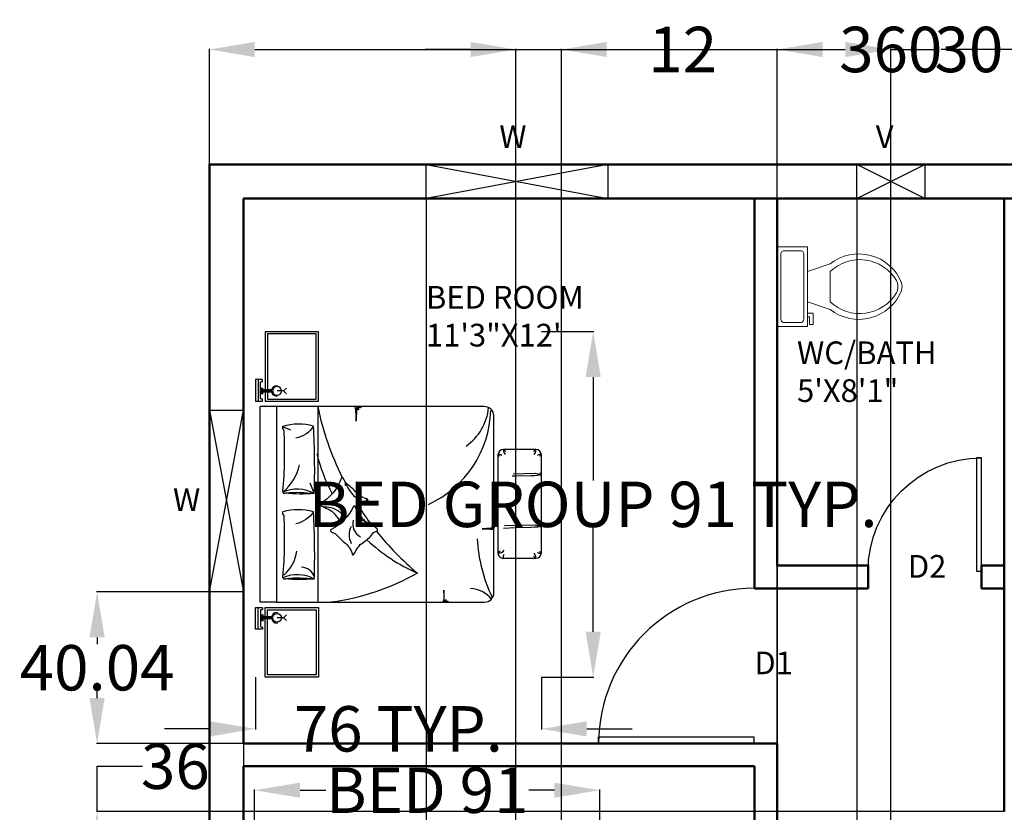
# Model space of a CAD drawing. Units: inches. Extents: x -77 to 516, y -119 to 536.
# Tile 7 of 11: x -36 to 224, y 323 to 533. Entities that reach past the tile are written whole.
import ezdxf

# ---------------------------------------------------------------- set-up
doc = ezdxf.new("R2010")
doc.units = ezdxf.units.IN
doc.header["$MEASUREMENT"] = 0
for name, color, linetype, lineweight in [('A-ANNO-DIMS', 2, 'Continuous', 18), ('A-AREA-IDEN', 170, 'Continuous', 25), ('A-FLOR-FIXT', 9, 'Continuous', 18), ('doors', 6, 'Continuous', 25), ('furniture', 119, 'Continuous', 18), ('text', 170, 'Continuous', 18), ('walls', 40, 'Continuous', 50), ('windows', 1, 'Continuous', 25)]:
    doc.layers.add(name, color=color, linetype=linetype, lineweight=lineweight)
for name, color, linetype in [('CEIL', 4, 'Continuous'), ('ELEC', 4, 'Continuous'), ('FUR', 42, 'Continuous'), ('wood', 26, 'Continuous')]:
    doc.layers.add(name, color=color, linetype=linetype)
doc.styles.get("Standard").update_dxf_attribs({"font": 'arial.ttf'})
doc.dimstyles.get("Standard").update_dxf_attribs({"dimtxt": 12, "dimasz": 12, "dimexe": 0.18, "dimexo": 0.0625, "dimgap": 0.09, "dimtad": 0, "dimtih": 1, "dimtoh": 1, "dimdec": 1, "dimzin": 0, "dimdsep": 46, "dimlunit": 4, "dimtxsty": 'Standard', "dimcen": 0.09, "dimadec": 0, "dimazin": 0, "dimtfac": 1, "dimtdec": 1, "dimtofl": 0, "dimtmove": 0, "dimatfit": 3, "dimfxl": 1, "dimtolj": 1, "dimtzin": 0, "dimarcsym": 0})

# ---------------------------------------------------------------- blocks, each defined once
blk = doc.blocks.new('*U2')
for p, q in [((0, 0), (0, -6)), ((40, 0), (40, -6))]:
    blk.add_line(p, q)
blk.add_lwpolyline([(0, 0), (0, 40), (1.75, 40), (1.75, 0)], close=True)
blk.add_arc((0, 0), 40, 0, 90)
blk = doc.blocks.new('*X12')
at = {"color": 0}
for p, q in [((3155.9, 8182.9), (3155.9, 8182.9)), ((3147.8, 8143.4), (3147.8, 8143.4)), ((3209.5, 8023.9), (3209.5, 8023.9)), ((3251.6, 7997), (3251.6, 7997)), ((3283, 8049.6), (3283, 8049.6)), ((3154.1, 7950.7), (3154.1, 7950.7))]:
    blk.add_line(p, q, dxfattribs=at)
blk = doc.blocks.new('*X11')
at = {"color": 0}
for p, q in [((3155.9, 8182.9), (3155.9, 8182.9)), ((3139.8, 7939.7), (3139.8, 7939.7))]:
    blk.add_line(p, q, dxfattribs=at)
blk = doc.blocks.new('*X10')
at = {"color": 0}
for p, q in [((3155.9, 8182.9), (3155.9, 8182.9)), ((3139.8, 7939.7), (3139.8, 7939.7))]:
    blk.add_line(p, q, dxfattribs=at)
blk = doc.blocks.new('*X9')
at = {"color": 0}
for p, q in [((3163, 7776.2), (3163, 7776.2)), ((3422.2, 7761.3), (3422.2, 7761.3)), ((3236.2, 7675.7), (3236.2, 7675.7)), ((3244.3, 7698.6), (3244.3, 7698.6)), ((3340.3, 7689.4), (3340.3, 7689.4))]:
    blk.add_line(p, q, dxfattribs=at)
blk = doc.blocks.new('BED1')
for p, q in [((0, -1000), (0, 800)), ((150, 800), (0, 800)), ((150, 800), (150, -1000)), ((2058.7, 800), (150, 800)), ((528, 800), (528, -1000)), ((211.8, 614.9), (277.5, 585.4)), ((2537.2, 404.9), (2237.2, 404.9)), ((2187.2, 354.9), (2187.2, -545.1)), ((2587.2, -545.1), (2587.2, 354.9)), ((2582, 188.1), (2565.4, 174.8)), ((2566.3, 178.5), (2565.2, 177.4)), ((2565.4, 174.8), (2585.7, 165.4)), ((2566.3, -296.8), (2565.2, -297.9)), ((2582, -287.1), (2565.4, -300.5)), ((2565.4, -300.5), (2585.7, -309.9)), ((2237.2, -595.1), (2537.2, -595.1)), ((150, -1000), (0, -1000)), ((150, -1000), (2063.5, -1000))]:
    blk.add_line(p, q)
for points in [[(934, 797.9), (930.9, 797.7), (928.3, 797.4), (926.3, 796.9), (924.9, 796.3), (923.8, 795.6), (923.1, 794.8), (922.7, 793.8), (922.5, 792.7), (922.4, 791.5), (922.5, 790.3), (922.6, 789.2), (922.6, 788.3), (922.6, 787.6), (922.4, 787.3), (922, 787.4), (921.4, 787.9), (920.6, 788.9), (919.5, 790.2), (918.4, 791.6), (917.1, 793.1), (915.9, 794.6), (914.6, 796), (913.3, 797.1), (912.2, 797.9), (911.1, 798.3), (910.1, 798.4), (909.2, 798), (908.3, 797.1), (907.5, 795.8), (906.8, 793.9), (906, 791.4), (905.4, 788.5), (904.8, 785.2), (904.2, 781.7), (903.7, 778.4), (903.2, 775.4), (902.8, 772.9), (902.5, 771.3), (902.3, 770.6), (902.1, 771.2), (902, 772.8), (901.8, 775.2), (901.7, 778.1), (901.5, 781.5), (901.2, 785), (900.8, 788.4), (900.2, 791.5), (899.5, 794.1), (898.6, 796.2), (897.6, 797.9), (896.5, 799.2), (895.3, 800), (894.1, 800.5), (893, 800.7), (891.9, 800.5), (890.9, 800.1), (890, 799), (889.1, 797.1), (888.3, 794), (887.6, 789.3), (886.9, 782.9), (886.2, 774.2), (885.5, 763.1), (884.8, 749.5), (884.2, 734.2), (883.6, 718.3), (883, 702.8), (882.5, 688.8), (882, 677.5), (881.7, 669.8), (881.5, 666.9), (881.3, 669.4), (881.3, 676.7), (881.3, 687.8), (881.2, 701.5), (881.1, 716.8), (880.8, 732.6), (880.2, 748), (879.4, 761.8), (878.3, 773.2), (876.9, 782.2), (875.1, 789.2), (872.9, 794.4), (870.3, 798), (869, 799)], [(2150, -913.5), (2150, 723.2)], [(2327.6, 182.3), (2530, 185.9), (2550.8, 181.9), (2561.7, 179), (2566, 176.7), (2566.9, 174.4), (2566.3, 171.9), (2562, 169.2), (2550.3, 166.5), (2527.7, 163.9), (2490.6, 161.8), (2345.5, 160.2), (2317.8, 158.5)], [(494.7, 3.1), (458.9, 95.3)], [(2149.7, -259.9), (2150, -268.4), (2150.1, -274.1), (2150.1, -278.1), (2150, -281.4), (2149.8, -284), (2149.5, -286.1), (2149.1, -287.8), (2148.7, -289), (2148.1, -289.9), (2147.4, -290.5), (2146.6, -290.8), (2145.6, -291), (2144.6, -291), (2143.6, -291), (2142.7, -290.9), (2141.9, -290.9), (2141.4, -290.9), (2141.1, -291), (2141.2, -291.4), (2141.7, -291.9), (2142.5, -292.6), (2143.5, -293.4), (2144.7, -294.4), (2146, -295.4), (2147.2, -296.5), (2148.4, -297.6), (2149.3, -298.6), (2150, -299.6), (2150.3, -300.5), (2150.4, -301.3), (2150, -302.1), (2149.3, -302.8), (2148.2, -303.5), (2146.6, -304.1), (2144.6, -304.7), (2142.1, -305.2), (2139.3, -305.7), (2136.5, -306.2), (2133.7, -306.6), (2131.2, -307), (2129.2, -307.3), (2127.8, -307.6), (2127.3, -307.8), (2127.7, -308), (2129, -308.1), (2131, -308.2), (2133.5, -308.3), (2136.3, -308.5), (2139.2, -308.7), (2142, -309), (2144.6, -309.5), (2146.8, -310.1), (2148.6, -310.9), (2150, -311.7), (2151, -312.7), (2151.7, -313.6), (2152.1, -314.6), (2152.3, -315.6), (2152.2, -316.5), (2151.8, -317.3), (2150.9, -318.1), (2149.3, -318.8), (2146.7, -319.4), (2142.8, -320), (2137.4, -320.6), (2130.2, -321.2), (2121, -321.8), (2109.7, -322.3), (2096.9, -322.9), (2083.6, -323.4), (2070.7, -323.9), (2059.1, -324.3), (2049.6, -324.7), (2043.2, -325), (2040.8, -325.2), (2042.9, -325.3), (2049, -325.3), (2058.2, -325.3), (2069.6, -325.4), (2082.3, -325.5), (2095.6, -325.8), (2108.4, -326.2), (2119.9, -326.8), (2129.4, -327.8), (2136.9, -329), (2142.7, -330.5), (2147, -332.3), (2150, -334.4), (2150.9, -335.6)], [(2246.5, -294.4), (2530, -289.4), (2550.8, -293.4), (2561.7, -296.3), (2566, -298.6), (2566.9, -300.8), (2566.3, -303.4), (2562, -306.1), (2550.3, -308.8), (2527.7, -311.3), (2490.6, -313.5), (2345.5, -315), (2238.6, -321.8)], [(1733.7, -998.3), (1731.1, -998.1), (1729, -997.8), (1727.4, -997.4), (1726.1, -997), (1725.2, -996.4), (1724.7, -995.7), (1724.3, -994.8), (1724.1, -993.9), (1724.1, -992.9), (1724.1, -991.9), (1724.2, -991), (1724.2, -990.2), (1724.2, -989.7), (1724.1, -989.4), (1723.8, -989.5), (1723.2, -990), (1722.5, -990.8), (1721.7, -991.8), (1720.7, -993), (1719.7, -994.3), (1718.6, -995.5), (1717.5, -996.6), (1716.5, -997.6), (1715.5, -998.3), (1714.6, -998.6), (1713.8, -998.6), (1713, -998.3), (1712.3, -997.6), (1711.7, -996.5), (1711, -994.9), (1710.4, -992.9), (1709.9, -990.4), (1709.4, -987.6), (1708.9, -984.8), (1708.5, -982), (1708.1, -979.5), (1707.8, -977.4), (1707.5, -976.1), (1707.3, -975.5), (1707.1, -976), (1707, -977.3), (1706.9, -979.3), (1706.8, -981.8), (1706.7, -984.6), (1706.4, -987.5), (1706.1, -990.3), (1705.6, -992.9), (1705, -995.1), (1704.2, -996.9), (1703.4, -998.3), (1702.4, -999.3), (1701.5, -1000), (1700.5, -1000.4), (1699.6, -1000.6), (1698.7, -1000.4), (1697.8, -1000.1), (1697, -999.2), (1696.3, -997.6), (1695.7, -995), (1695.1, -991.1), (1694.5, -985.7), (1693.9, -978.5), (1693.3, -969.3), (1692.8, -957.9), (1692.2, -945.2), (1691.7, -931.9), (1691.2, -919), (1690.8, -907.4), (1690.4, -897.9), (1690.1, -891.5), (1689.9, -889.1), (1689.8, -891.2), (1689.8, -897.3), (1689.8, -906.5), (1689.7, -917.9), (1689.6, -930.6), (1689.4, -943.8), (1688.9, -956.6), (1688.3, -968.1), (1687.3, -977.6), (1686.1, -985.2), (1684.6, -991), (1682.8, -995.3), (1680.7, -998.3), (1679.6, -999.2)]]:
    blk.add_lwpolyline(points)
for points in [[(489.2, 619.6, 0.144019), (207.6, 617.9, 0.248643)], [(205.5, 619.6, 0.267769), (215.1, 582.4, -0.037739), (204.3, 21.8, 0.684696), (236.7, 5.5, -0.060702), (497.2, 0.1, -0.046649), (225.9, 3.1, -1.318436)], [(497.2, 0.1, 0.021276), (489.2, 619.6, -0.206383), (326.6, 509.4, 0.237198)], [(211.8, 12.8, 0.143972), (361.6, 262.9, 1.292232)], [(886.4, -150, -0.069098), (985, -66.5, 0.658965), (982.1, -48.7, -0.049789), (927.4, -29, -0.103757), (896.6, -5.4, 0.055725), (800.9, 83.3, -0.11866), (782.7, 104.9, 0.016811), (761.6, 143.9, 0.70791), (748.3, 144, -0.16964), (551.9, -96.6, 0.664036), (554, -110.7, 0.023706), (627, -144.7, -0.134834), (683.2, -188, 0.012748), (746.3, -267.4)], [(205.5, -168.2, 0.267769), (215.1, -205.4, -0.037739), (204.3, -766, 0.684696), (236.7, -782.3, -0.060702), (497.2, -787.7, -0.046649), (225.9, -784.7, -1.318436)], [(489.2, -168.2, 0.144019), (207.6, -169.9, 0.248643)], [(497.2, -787.7, 0.021276), (489.2, -168.2, -0.206383), (326.6, -278.4, 0.237198)], [(969.1, -259.1, 0.263265), (936.3, -236.9, -0.026108), (909.2, -233.2, 0.027613), (945.1, -234.2, -0.089259), (872.7, -120, 0.662242), (857.6, -119.3, -0.162037), (651.8, -332.7, 0.676499), (654, -354.5, -0.160513), (722.9, -401.5, 0.07473), (773.5, -450.3, -0.187721), (845.5, -559.9, 0.70791), (858.8, -561.4, -0.010003), (898.6, -497.3, -0.113819), (947.3, -450.2, 0.099539), (1032.5, -372.4, -0.173425), (1070.9, -346.4, 0.589988), (1076.2, -326.1, 0.137312), (923.9, -245.9, 0.137312)], [(1446, -733.4, -0.095039), (652.8, -1001.7)]]:
    blk.add_lwpolyline(points, format="xyb")
for centre, radius, start, end in [((3208.8, 1363.3), 2739.4, 191.86791, 206.32469), ((1138.6, 793.9), 983.2, 294.60777, 358.30329), ((1608.1, 842.5), 496.3, 305.19014, 354.02057), ((2062.7, 713.7), 86.5, 0, 93.53765), ((2098.7, 754.7), 1625, 193.90497, 207.81692), ((2237.2, 354.9), 50, 90, 180), ((2321.1, 409.7), 84.5, 185.61958, 217.13957), ((2227.5, 373.5), 32.8, 17.83305, 72.80048), ((2546.9, 373.5), 32.8, 107.19952, 162.16695), ((2453.3, 409.7), 84.5, 322.86043, 354.38042), ((2537.2, 354.9), 50, 0, 90), ((2201.9, 323.3), 34.8, 50.8413, 114.9586), ((2212.2, 381.5), 36.5, 226.80948, 258.3841), ((2572.5, 323.3), 34.8, 65.0414, 129.1587), ((2562.2, 381.5), 36.5, 281.6159, 313.19052), ((751.8, 88.7), 34.9, 336.83517, 27.72181), ((684.2, 86), 100.3, 353.675, 10.88198), ((1074.1, 198.8), 306.1, 197.86019, 241.51221), ((341.4, -277.7), 318.5, 60.71255, 115.00895), ((983.7, -79.5), 20.8, 73.79673, 130.45661), ((978.5, -68.6), 14.3, 39.7097, 85.9506), ((602.5, -324), 198.6, 43.20348, 95.05559), ((3208.8, 1363.3), 2739.4, 212.93136, 216.95099), ((981.1, -281.8), 131.1, 164.0372, 243.45361), ((980, -379), 163.4, 152.61037, 209.36102), ((3208.8, 1363.3), 2739.4, 218.63292, 229.94485), ((2098.7, 754.7), 1625, 226.58872, 246.3156), ((3402.5, -342.9), 1408.5, 182.99169, 205.68187), ((-34.4, -471.2), 376.5, 312.01178, 350.96348), ((2178, -513.5), 33, 286.18268, 338.13858), ((2188.1, -476.2), 73, 269.45125, 322.80265), ((2572.5, -513.6), 34.8, 230.8413, 294.9586), ((2562.2, -571.8), 36.5, 46.80948, 78.3841), ((2237.2, -545.1), 50, 180, 270), ((2271.1, -580.9), 35.8, 148.90546, 197.55407), ((2546.9, -563.8), 32.8, 197.83305, 252.80048), ((2453.3, -600), 84.5, 5.61958, 37.13957), ((2537.2, -545.1), 50, 270, 0), ((375.7, -807.4), 128.2, 17.40732, 88.51286), ((341.4, -1065.5), 318.5, 60.71255, 115.00895), ((1929.1, -1126), 250.5, 37.85533, 88.44053), ((2063.5, -913.5), 86.5, 270, 0)]:
    blk.add_arc(centre, radius, start, end)
for name in ['*X11', '*X10', '*X12', '*X9']:
    blk.add_blockref(name, (-2425.3, -8101.4))
blk = doc.blocks.new('APLIQ')
at = {"layer": 'ELEC'}
for p, q in [((0, 0.2), (-0.0261, 0.2261)), ((0, 0.2), (0.0261, 0.2261)), ((0, 0.2), (0, 0.14)), ((-0.05, 0.14), (-0.04, 0.14)), ((0.04, 0.14), (0.05, 0.14)), ((-0.03, 0.01), (0.03, 0.01)), ((-0.03, 0), (0.03, 0)), ((-0.01, 0.09), (-0.01, 0.01)), ((0, 0.09), (0, 0)), ((0.01, 0.09), (0.01, 0.01))]:
    blk.add_line(p, q, dxfattribs=at)
blk.add_circle((0, 0.14), 0.04, dxfattribs=at)
blk.add_arc((0, 0.14), 0.05, 180, 0, dxfattribs=at)
blk = doc.blocks.new('A$C68AE1801')
at = {"layer": 'FUR'}
for points in [[(2.5416, 3.18), (2.5416, 2.54), (2.0516, 2.54), (2.0516, 3.18)], [(2.5216, 3.16), (2.5216, 2.56), (2.0716, 2.56), (2.0716, 3.16)], [(2.5416, 0), (2.5416, 0.64), (2.0516, 0.64), (2.0516, 0)], [(2.5216, 0.02), (2.5216, 0.62), (2.0716, 0.62), (2.0716, 0.02)]]:
    blk.add_lwpolyline(points, close=True, dxfattribs=at)
at = {"layer": 'wood'}
for p, q in [((2.6057, 2.74), (2.6057, 2.54)), ((2.6057, 0.44), (2.6057, 0.64))]:
    blk.add_line(p, q, dxfattribs=at)
for points in [[(2.5657, 2.728), (2.5657, 2.732, -0.414214), (2.5737, 2.74), (2.6321, 2.74), (2.6321, 2.54), (2.5737, 2.54, -0.414214), (2.5657, 2.548), (2.5657, 2.552, -0.414214), (2.5737, 2.56), (2.5777, 2.56, 0.414214), (2.5857, 2.568), (2.5857, 2.712, 0.414214), (2.5777, 2.72), (2.5737, 2.72, -0.414214)], [(2.5657, 0.452), (2.5657, 0.448, 0.414214), (2.5737, 0.44), (2.6321, 0.44), (2.6321, 0.64), (2.5737, 0.64, 0.414214), (2.5657, 0.632), (2.5657, 0.628, 0.414214), (2.5737, 0.62), (2.5777, 0.62, -0.414214), (2.5857, 0.612), (2.5857, 0.468, -0.414214), (2.5777, 0.46), (2.5737, 0.46, 0.414214)]]:
    blk.add_lwpolyline(points, format="xyb", close=True, dxfattribs=at)
at = {"layer": 'CEIL', "rotation": 90}
blk.add_blockref('APLIQ', (2.5736, 2.634), dxfattribs=at)
at = {"layer": 'CEIL', "xscale": -1, "rotation": 90}
blk.add_blockref('APLIQ', (2.5736, 0.546), dxfattribs=at)
at = {"layer": 'FUR', "xscale": 0.001, "yscale": 0.001, "zscale": 0.001, "rotation": 180}
blk.add_blockref('BED1', (2.5872, 1.49), dxfattribs=at)
blk = doc.blocks.new('*U16')
for p, q in [((9.5, -6), (9.5, -2)), ((-10, -8.5), (-8, -8.5)), ((-10, -9.5), (-10, -8.5)), ((-7, -9.5), (-10, -9.5)), ((-8, -8.5), (-8, -8)), ((-7, -8), (-7, -9.5)), ((-4, -8), (-6, -14)), ((4, -8), (6, -14)), ((4, -14), (-4, -14))]:
    blk.add_line(p, q)
blk.add_lwpolyline([(10.5, -8), (10.5, 0), (-10.5, 0), (-10.5, -8)], close=True)
for points in [[(-9.5, -2), (-9.5, -6)], [(8.5, -1), (-8.5, -1)], [(-8.5, -7), (8.5, -7)]]:
    blk.add_lwpolyline(points)
for centre, radius, start, end in [((-8.62, -1.88), 0.884, 81.8699, 188.1301), ((8.62, -1.88), 0.884, 351.8699, 98.1301), ((-8.62, -6.12), 0.884, 171.8699, 278.1301), ((8.62, -6.12), 0.884, 261.8699, 8.1301), ((3.52, -21.58), 12.17, 141.4691, 247.9714), ((4.2, -21.82), 11.33, 136.3677, 238.9468), ((-3.52, -21.58), 12.17, 292.0284, 38.5307), ((-4.2, -21.82), 11.33, 301.053, 43.6321), ((0, -27.88), 4, 245.7318, 294.2682), ((0, -29), 4, 254.8605, 285.1395)]:
    blk.add_arc(centre, radius, start, end)
blk = doc.blocks.new('WIN-48IN')
for p, q in [((0, 0), (9, 48)), ((0, 48), (9, 0))]:
    blk.add_line(p, q)
blk.add_lwpolyline([(0, 48), (9, 48), (9, 0), (0, 0)], close=True)
blk = doc.blocks.new('WIN-18IN')
for p, q in [((18, 0), (0, 9)), ((0, 0), (18, 9))]:
    blk.add_line(p, q)
blk.add_lwpolyline([(0, 9), (18, 9), (18, 0), (0, 0)], close=True)
blk = doc.blocks.new('*D26')
at = {"layer": 'A-ANNO-DIMS', "color": 0, "lineweight": -2, "transparency": 16777216}
for p, q in [((101.52, 450.4), (115.33, 450.4)), ((115.15, 438.4), (115.15, 411.07)), ((115.15, 371.14), (115.15, 398.47)), ((101.52, 359.14), (115.33, 359.14))]:
    blk.add_line(p, q, dxfattribs=at)
at = {"layer": 'A-ANNO-DIMS', "color": 0, "transparency": 16777216}
for points in [[(113.15, 438.4), (117.15, 438.4), (115.15, 450.4)], [(113.15, 371.14), (117.15, 371.14), (115.15, 359.14)]]:
    blk.add_solid(points, dxfattribs=at)
at = {"layer": 'Defpoints', "color": 0, "transparency": 16777216}
for p in [(101.46, 450.4), (101.46, 359.14), (115.15, 359.14)]:
    blk.add_point(p, dxfattribs=at)
at = {"layer": 'A-ANNO-DIMS', "color": 0, "transparency": 16777216, "insert": (115.15, 404.77), "char_height": 12, "attachment_point": 5}
blk.add_mtext('\\A1;BED GROUP 91 TYP.', dxfattribs=at)
blk = doc.blocks.new('*D27')
at = {"layer": 'A-ANNO-DIMS', "color": 0, "lineweight": -2, "transparency": 16777216}
for p, q in [((25.93, 359.08), (25.93, 345.28)), ((101.46, 359.08), (101.46, 345.28)), ((13.93, 345.46), (1.93, 345.46)), ((113.46, 345.46), (125.46, 345.46))]:
    blk.add_line(p, q, dxfattribs=at)
at = {"layer": 'A-ANNO-DIMS', "color": 0, "transparency": 16777216}
for points in [[(13.93, 347.46), (13.93, 343.46), (25.93, 345.46)], [(113.46, 347.46), (113.46, 343.46), (101.46, 345.46)]]:
    blk.add_solid(points, dxfattribs=at)
at = {"layer": 'Defpoints', "color": 0, "transparency": 16777216}
for p in [(25.93, 359.14), (101.46, 359.14), (25.93, 345.46)]:
    blk.add_point(p, dxfattribs=at)
at = {"layer": 'A-ANNO-DIMS', "color": 0, "transparency": 16777216, "insert": (63.69, 345.46), "char_height": 12, "attachment_point": 5}
blk.add_mtext('\\A1;76 TYP.', dxfattribs=at)
blk = doc.blocks.new('*D28')
at = {"layer": 'A-ANNO-DIMS', "color": 0, "lineweight": -2, "transparency": 16777216}
for p, q in [((25.71, 315.63), (25.71, 329.43)), ((37.71, 329.25), (44.48, 329.25)), ((104.89, 329.25), (98.13, 329.25)), ((116.89, 315.63), (116.89, 329.43))]:
    blk.add_line(p, q, dxfattribs=at)
at = {"layer": 'A-ANNO-DIMS', "color": 0, "transparency": 16777216}
for points in [[(37.71, 331.25), (37.71, 327.25), (25.71, 329.25)], [(104.89, 331.25), (104.89, 327.25), (116.89, 329.25)]]:
    blk.add_solid(points, dxfattribs=at)
at = {"layer": 'Defpoints', "color": 0, "transparency": 16777216}
for p in [(25.71, 329.25), (25.71, 315.57), (116.89, 315.57)]:
    blk.add_point(p, dxfattribs=at)
at = {"layer": 'A-ANNO-DIMS', "color": 0, "transparency": 16777216, "insert": (71.3, 329.25), "char_height": 12, "attachment_point": 5}
blk.add_mtext('\\A1;BED 91', dxfattribs=at)
blk = doc.blocks.new('*D36')
at = {"layer": 'A-ANNO-DIMS', "color": 0, "lineweight": -2, "transparency": 16777216}
for p, q in [((13.75, 494.65), (13.75, 525.13)), ((25.75, 524.95), (180.43, 524.95)), ((361.75, 524.95), (207.07, 524.95)), ((373.75, 494.65), (373.75, 525.13))]:
    blk.add_line(p, q, dxfattribs=at)
at = {"layer": 'A-ANNO-DIMS', "color": 0, "transparency": 16777216}
for points in [[(25.75, 526.95), (25.75, 522.95), (13.75, 524.95)], [(361.75, 526.95), (361.75, 522.95), (373.75, 524.95)]]:
    blk.add_solid(points, dxfattribs=at)
at = {"layer": 'Defpoints', "color": 0, "transparency": 16777216}
for p in [(373.75, 524.95), (13.75, 494.59), (373.75, 494.59)]:
    blk.add_point(p, dxfattribs=at)
at = {"layer": 'A-ANNO-DIMS', "color": 0, "transparency": 16777216, "insert": (193.75, 524.95), "char_height": 12, "attachment_point": 5}
blk.add_mtext('\\A1;360', dxfattribs=at)
blk = doc.blocks.new('*D39')
at = {"layer": 'A-ANNO-DIMS', "color": 0, "lineweight": -2, "transparency": 16777216}
for p, q in [((22.75, 485.53), (22.75, -111.24)), ((71.05, 485.53), (71.05, -111.24)), ((34.75, -111.06), (59.05, -111.06)), ((71.05, -111.06), (83.05, -111.06))]:
    blk.add_line(p, q, dxfattribs=at)
at = {"layer": 'A-ANNO-DIMS', "color": 0, "transparency": 16777216}
for points in [[(34.75, -109.06), (34.75, -113.06), (22.75, -111.06)], [(59.05, -109.06), (59.05, -113.06), (71.05, -111.06)]]:
    blk.add_solid(points, dxfattribs=at)
at = {"layer": 'Defpoints', "color": 0, "transparency": 16777216}
for p in [(22.75, 485.59), (71.05, 485.59), (71.05, -111.06)]:
    blk.add_point(p, dxfattribs=at)
at = {"layer": 'A-ANNO-DIMS', "color": 0, "transparency": 16777216, "insert": (108.33, -111.06), "char_height": 12, "attachment_point": 5}
blk.add_mtext('\\A1;48.295', dxfattribs=at)
blk = doc.blocks.new('*D40')
at = {"layer": 'A-ANNO-DIMS', "color": 0, "lineweight": -2, "transparency": 16777216}
for p, q in [((163.750061, 485.5259), (163.750061, -111.2416)), ((184.750061, 485.5259), (184.750061, -111.2416)), ((151.750061, -111.0616), (139.750061, -111.0616)), ((196.750061, -111.0616), (208.750061, -111.0616))]:
    blk.add_line(p, q, dxfattribs=at)
at = {"layer": 'A-ANNO-DIMS', "color": 0, "transparency": 16777216}
for points in [[(151.750061, -109.0616), (151.750061, -113.0616), (163.750061, -111.0616)], [(196.750061, -109.0616), (196.750061, -113.0616), (184.750061, -111.0616)]]:
    blk.add_solid(points, dxfattribs=at)
at = {"layer": 'Defpoints', "color": 0, "transparency": 16777216}
for p in [(163.750061, 485.5884), (184.750061, 485.5884), (184.750061, -111.0616)]:
    blk.add_point(p, dxfattribs=at)
at = {"layer": 'A-ANNO-DIMS', "color": 0, "transparency": 16777216, "insert": (174.250061, -111.0616), "char_height": 12, "attachment_point": 5}
blk.add_mtext('\\A1;21', dxfattribs=at)
blk = doc.blocks.new('*D44')
at = {"layer": 'A-ANNO-DIMS', "color": 0, "lineweight": -2, "transparency": 16777216}
for p, q in [((22.69, 381.63), (-16.08, 381.63)), ((-15.9, 369.63), (-15.9, 367.82)), ((-15.9, 353.59), (-15.9, 355.39)), ((22.69, 341.59), (-16.08, 341.59))]:
    blk.add_line(p, q, dxfattribs=at)
at = {"layer": 'A-ANNO-DIMS', "color": 0, "transparency": 16777216}
for points in [[(-17.9, 369.63), (-13.9, 369.63), (-15.9, 381.63)], [(-17.9, 353.59), (-13.9, 353.59), (-15.9, 341.59)]]:
    blk.add_solid(points, dxfattribs=at)
at = {"layer": 'Defpoints', "color": 0, "transparency": 16777216}
for p in [(-15.9, 381.63), (22.75, 381.63), (22.75, 341.59)]:
    blk.add_point(p, dxfattribs=at)
at = {"layer": 'A-ANNO-DIMS', "color": 0, "transparency": 16777216, "insert": (-15.9, 361.61), "char_height": 12, "attachment_point": 5}
blk.add_mtext('\\A1;40.04', dxfattribs=at)
blk = doc.blocks.new('*D46')
at = {"layer": 'A-ANNO-DIMS', "color": 0, "lineweight": -2, "transparency": 16777216}
for p, q in [((-15.9, 323.59), (-15.9, 335.59)), ((-15.9, 335.59), (-3.9, 335.59)), ((223.69, 323.59), (-16.08, 323.59)), ((-15.9, 299.59), (-15.9, 311.59)), ((223.69, 287.59), (-16.08, 287.59))]:
    blk.add_line(p, q, dxfattribs=at)
at = {"layer": 'A-ANNO-DIMS', "color": 0, "transparency": 16777216}
for points in [[(-17.9, 311.59), (-13.9, 311.59), (-15.9, 323.59)], [(-17.9, 299.59), (-13.9, 299.59), (-15.9, 287.59)]]:
    blk.add_solid(points, dxfattribs=at)
at = {"layer": 'Defpoints', "color": 0, "transparency": 16777216}
for p in [(-15.9, 323.59), (223.75, 323.59), (223.75, 287.59)]:
    blk.add_point(p, dxfattribs=at)
at = {"layer": 'A-ANNO-DIMS', "color": 0, "transparency": 16777216, "insert": (4.78, 335.59), "char_height": 12, "attachment_point": 5}
blk.add_mtext('\\A1;36', dxfattribs=at)
blk = doc.blocks.new('*D53')
at = {"layer": 'A-ANNO-DIMS', "color": 0, "lineweight": -2, "transparency": 16777216}
for p, q in [((163.75, 95.65), (163.75, 525.13)), ((175.75, 524.95), (181.75, 524.95)), ((193.75, 95.65), (193.75, 525.13)), ((193.75, 524.95), (205.75, 524.95))]:
    blk.add_line(p, q, dxfattribs=at)
at = {"layer": 'A-ANNO-DIMS', "color": 0, "transparency": 16777216}
for points in [[(175.75, 526.95), (175.75, 522.95), (163.75, 524.95)], [(181.75, 526.95), (181.75, 522.95), (193.75, 524.95)]]:
    blk.add_solid(points, dxfattribs=at)
at = {"layer": 'Defpoints', "color": 0, "transparency": 16777216}
for p in [(193.75, 524.95), (163.75, 95.59), (193.75, 95.59)]:
    blk.add_point(p, dxfattribs=at)
at = {"layer": 'A-ANNO-DIMS', "color": 0, "transparency": 16777216, "insert": (214.41, 524.95), "char_height": 12, "attachment_point": 5}
blk.add_mtext('\\A1;30', dxfattribs=at)
blk = doc.blocks.new('*D54')
at = {"layer": 'A-ANNO-DIMS', "color": 0, "lineweight": -2, "transparency": 16777216}
for p, q in [((82.75, 524.95), (70.75, 524.95)), ((94.75, 120.65), (94.75, 525.13)), ((106.75, 120.65), (106.75, 525.13)), ((118.75, 524.95), (130.75, 524.95))]:
    blk.add_line(p, q, dxfattribs=at)
at = {"layer": 'A-ANNO-DIMS', "color": 0, "transparency": 16777216}
for points in [[(82.75, 526.95), (82.75, 522.95), (94.75, 524.95)], [(118.75, 526.95), (118.75, 522.95), (106.75, 524.95)]]:
    blk.add_solid(points, dxfattribs=at)
at = {"layer": 'Defpoints', "color": 0, "transparency": 16777216}
for p in [(106.75, 524.95), (94.75, 120.59), (106.75, 120.59)]:
    blk.add_point(p, dxfattribs=at)
at = {"layer": 'A-ANNO-DIMS', "color": 0, "transparency": 16777216, "insert": (138.81, 524.95), "char_height": 12, "attachment_point": 5}
blk.add_mtext('\\A1;12', dxfattribs=at)

msp = doc.modelspace()

# ---------------------------------------------------------------- linework, layer by layer
at = {"layer": 'walls'}
for p, q in [((364.7501, 485.5884), (22.7501, 485.5884)), ((22.7501, 485.5884), (22.7501, 341.5884)), ((157.7501, 485.5884), (157.7501, 382.5884)), ((163.7501, 485.5884), (163.7501, 431.5884)), ((223.7501, 485.5884), (223.7501, 431.5884)), ((223.7501, 485.5884), (223.7501, 431.5884)), ((163.7501, 431.5884), (163.7501, 388.5884)), ((223.7501, 431.5884), (223.7501, 323.5884)), ((223.7501, 425.5884), (223.7501, 323.5884)), ((187.7501, 388.5884), (163.7501, 388.5884)), ((187.7501, 388.5884), (187.7501, 382.5884)), ((223.7501, 388.5884), (217.7501, 388.5884)), ((217.7501, 388.5884), (217.7501, 382.5884)), ((187.7501, 382.5884), (157.7501, 382.5884)), ((223.7501, 382.5884), (217.7501, 382.5884)), ((163.7501, 341.5884), (22.7501, 341.5884)), ((163.7501, 341.5884), (163.7501, 245.5884)), ((157.7501, 335.5884), (22.7501, 335.5884)), ((22.7501, 335.5884), (22.7501, 23.5884)), ((157.7501, 335.5884), (157.7501, 245.5884))]:
    msp.add_line(p, q, dxfattribs=at)
msp.add_lwpolyline([(373.7501, 131.5884), (373.7501, 494.5884), (13.7501, 494.5884), (13.7501, 14.5884), (239.7501, 14.5884)], dxfattribs=at)

# ---------------------------------------------------------------- block references
at = {"layer": 'A-FLOR-FIXT', "rotation": 90}
msp.add_blockref('*U16', (163.7501, 462.2957), dxfattribs=at)
at = {"layer": 'doors', "xscale": -0.7499999999999992, "yscale": 0.7499999999999992, "zscale": 0.7499999999999992}
msp.add_blockref('*U2', (217.7501, 387.0884), dxfattribs=at)
at = {"layer": 'doors', "xscale": 1.025133417478691, "yscale": 1.025133417478691, "zscale": 1.025133417478691, "rotation": 90}
msp.add_blockref('*U2', (157.5993, 341.5884), dxfattribs=at)
at = {"layer": 'furniture', "xscale": 28.69583594835296, "yscale": 28.69583594835296, "zscale": 28.69583594835296, "rotation": 180}
msp.add_blockref('A$C68AE1801', (101.4593, 450.3969), dxfattribs=at)
at = {"layer": 'windows', "rotation": 270}
msp.add_blockref('WIN-48IN', (71.0456, 494.5885), dxfattribs=at)
at = {"layer": 'windows'}
for name, p in [('WIN-18IN', (184.75, 485.588)), ('WIN-48IN', (13.75, 381.626))]:
    msp.add_blockref(name, p, dxfattribs=at)

# ---------------------------------------------------------------- texts
at = {"layer": 'A-AREA-IDEN', "char_height": 6, "attachment_point": 1}
for s, insert in [('BED ROOM\\P11\'3"X12\'', (70.9694, 462.4771)), ('WC/BATH\\P5\'X8\'1"', (169.0007, 447.8176))]:
    msp.add_mtext_dynamic_manual_height_columns(s, width=105.041962, gutter_width=1, heights=[0], dxfattribs=dict(at, insert=insert))
at = {"layer": 'text', "char_height": 6, "attachment_point": 1}
for s, insert in [('W', (90.3498, 504.9353)), ('V ', (189.7745, 504.9353)), ('W', (4.1565, 408.9867)), ('D2', (198.2704, 391.3943)), ('D1', (157.729, 365.8953))]:
    msp.add_mtext_dynamic_manual_height_columns(s, width=105.041962, gutter_width=1, heights=[0], dxfattribs=dict(at, insert=insert))

# ---------------------------------------------------------------- dimensions: what is measured, and where the dimension line sits
at = {"layer": 'A-ANNO-DIMS'}
for base, p1, p2, override, picture, middle in [((373.7501, 524.9457), (13.7501, 494.5884), (373.7501, 494.5884), {"dimdec": 0, "dimlfac": 1, "dimrnd": 0, "dimzin": 0, "dimdsep": 46, "dimlunit": 2}, '*D36', (193.7501, 524.9457)), ((106.7501, 524.9457), (94.7501, 120.5884), (106.7501, 120.5884), {"dimdec": 0, "dimlfac": 1, "dimrnd": 0, "dimzin": 0, "dimdsep": 46, "dimlunit": 2}, '*D54', (138.8087, 524.9457)), ((193.7501, 524.9457), (163.7501, 95.5884), (193.7501, 95.5884), {"dimdec": 0, "dimlfac": 1, "dimrnd": 0, "dimzin": 0, "dimdsep": 46, "dimlunit": 2}, '*D53', (214.4103, 524.9457)), ((71.0451, -111.0616), (22.7501, 485.5884), (71.0451, 485.5884), {"dimdec": 3, "dimlfac": 1, "dimrnd": 0, "dimzin": 0, "dimdsep": 46, "dimlunit": 2}, '*D39', (108.3302, -111.0616)), ((184.7501, -111.0616), (163.7501, 485.5884), (184.7501, 485.5884), {"dimdec": 0, "dimlfac": 1, "dimrnd": 0, "dimzin": 0, "dimdsep": 46, "dimlunit": 2}, '*D40', (174.2501, -111.0616))]:
    dim = msp.add_linear_dim(base=base, p1=p1, p2=p2, dimstyle='Standard', override=override, dxfattribs=at)
    dim.commit()
    dim.dimension.update_dxf_attribs({"geometry": picture, "text_midpoint": middle})
for base, p1, p2, angle, text, picture, middle in [((115.1473, 359.1441), (101.4593, 450.3969), (101.4593, 359.1441), 270, 'BED GROUP <> TYP.', '*D26', (115.1473, 404.7705)), ((25.9277, 345.4562), (101.4593, 359.1441), (25.9277, 359.1441), 180, '<> TYP.', '*D27', (63.6935, 345.4562)), ((25.7144, 329.2459), (116.8925, 315.5692), (25.7144, 315.5692), 180, 'BED <>', '*D28', (71.3034, 329.2459))]:
    dim = msp.add_linear_dim(base=base, p1=p1, p2=p2, angle=angle, text=text, dimstyle='Standard', override={"dimdec": 0, "dimlfac": 1, "dimrnd": 0, "dimzin": 0, "dimdsep": 46, "dimlunit": 2}, dxfattribs=at)
    dim.commit()
    dim.dimension.update_dxf_attribs({"geometry": picture, "text_midpoint": middle})
for base, p1, p2, override, picture, middle in [((-15.8999, 381.6255), (22.7501, 341.5884), (22.7501, 381.6255), {"dimdec": 2, "dimlfac": 1, "dimrnd": 0, "dimzin": 0, "dimdsep": 46, "dimlunit": 2}, '*D44', (-15.8999, 361.607)), ((-15.8999, 323.5884), (223.7501, 287.5884), (223.7501, 323.5884), {"dimdec": 0, "dimlfac": 1, "dimrnd": 0, "dimzin": 0, "dimdsep": 46, "dimlunit": 2}, '*D46', (4.7767, 335.5884))]:
    dim = msp.add_linear_dim(base=base, p1=p1, p2=p2, angle=90, dimstyle='Standard', override=override, dxfattribs=at)
    dim.commit()
    dim.dimension.update_dxf_attribs({"geometry": picture, "text_midpoint": middle})

doc.saveas('drawing.dxf')
